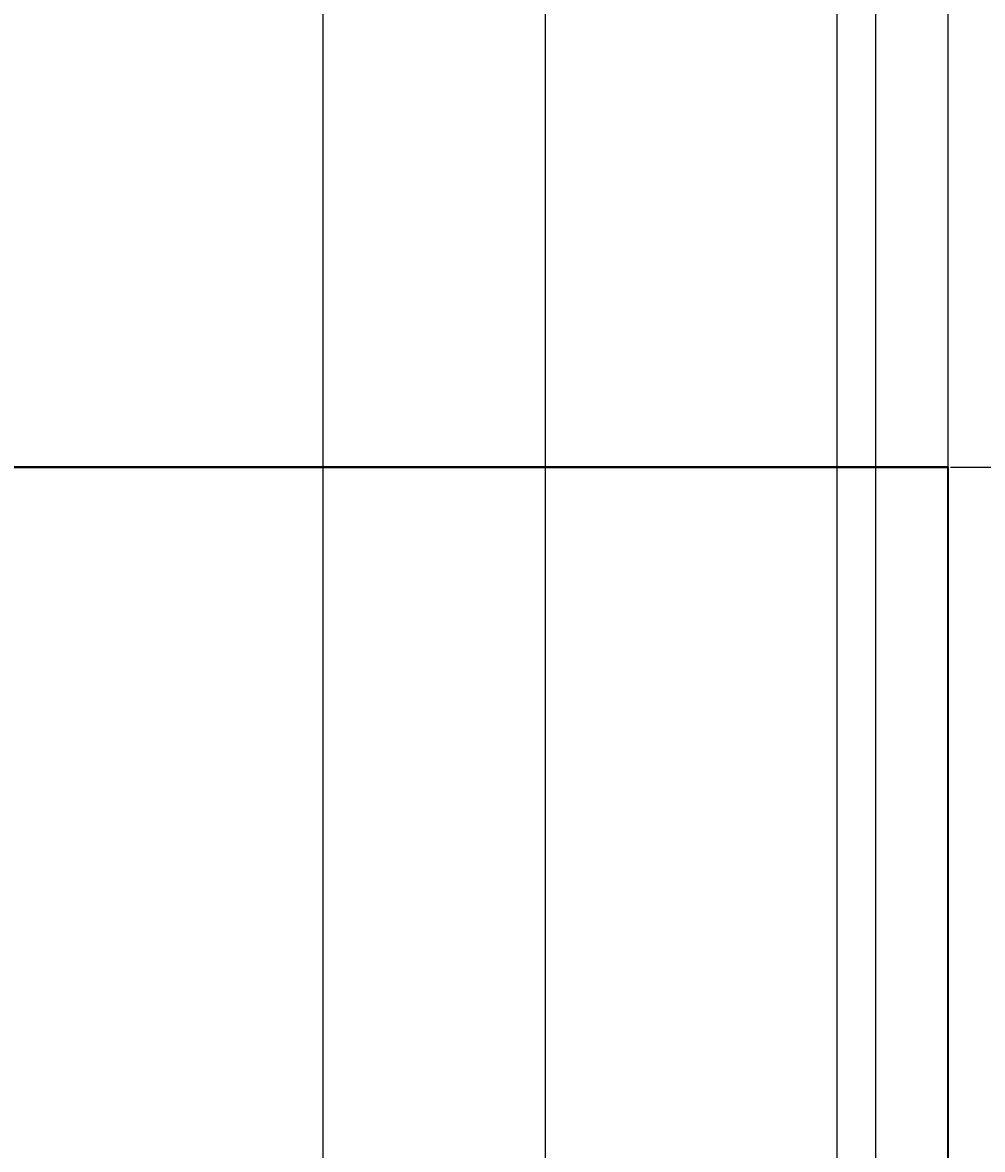
# Model space of a CAD drawing. Units: inches. Extents: x -6 to 289, y -8 to 323.
# Tile 95 of 107: x 222 to 248, y 229 to 259. Entities that reach past the tile are written whole.
import ezdxf

# ---------------------------------------------------------------- set-up
doc = ezdxf.new("R2010")
doc.units = ezdxf.units.IN
doc.header["$MEASUREMENT"] = 0
doc.layers.add('A-ANNO-DIMS', color=2, linetype='Continuous', lineweight=18)
doc.layers.add('A-ELEV', color=7, linetype='Continuous', lineweight=35)
doc.styles.get("Standard").update_dxf_attribs({"font": 'arial.ttf'})
doc.dimstyles.get("Standard").update_dxf_attribs({"dimtxt": 0.18, "dimasz": 0.18, "dimexe": 0.18, "dimexo": 0.0625, "dimgap": 0.09, "dimtad": 0, "dimtih": 1, "dimtoh": 1, "dimdec": 4, "dimzin": 0, "dimdsep": 46, "dimtxsty": 'Standard', "dimcen": 0.09, "dimadec": 0, "dimazin": 0, "dimtfac": 1, "dimtdec": 4, "dimtofl": 0, "dimtmove": 0, "dimatfit": 3, "dimfxl": 1, "dimtolj": 1, "dimtzin": 0, "dimarcsym": 0})

# ---------------------------------------------------------------- blocks, each defined once
blk = doc.blocks.new('*D13')
at = {"layer": 'A-ANNO-DIMS', "color": 0, "lineweight": -2, "transparency": 16777216}
for p, q in [((188.292, 226.951), (188.292, 322.969)), ((236.292, 226.951), (236.292, 322.969)), ((188.472, 322.789), (212.069, 322.789)), ((236.112, 322.789), (212.515, 322.789))]:
    blk.add_line(p, q, dxfattribs=at)
at = {"layer": 'A-ANNO-DIMS', "color": 0, "transparency": 16777216}
for points in [[(188.472, 322.819), (188.472, 322.759), (188.292, 322.789)], [(236.112, 322.819), (236.112, 322.759), (236.292, 322.789)]]:
    blk.add_solid(points, dxfattribs=at)
at = {"layer": 'Defpoints', "color": 0, "transparency": 16777216}
for p in [(236.292, 322.789), (188.292, 226.889), (236.292, 226.889)]:
    blk.add_point(p, dxfattribs=at)
at = {"layer": 'A-ANNO-DIMS', "color": 0, "transparency": 16777216, "insert": (212.292, 322.789), "char_height": 0.18, "attachment_point": 5}
blk.add_mtext('\\A1;48', dxfattribs=at)
blk = doc.blocks.new('*D14')
at = {"layer": 'A-ANNO-DIMS', "color": 0, "lineweight": -2, "transparency": 16777216}
for p, q in [((236.292, 226.951), (236.292, 322.969)), ((247.164, 162.411), (247.164, 322.969)), ((236.472, 322.789), (241.274, 322.789)), ((246.984, 322.789), (242.182, 322.789))]:
    blk.add_line(p, q, dxfattribs=at)
at = {"layer": 'A-ANNO-DIMS', "color": 0, "transparency": 16777216}
for points in [[(236.472, 322.819), (236.472, 322.759), (236.292, 322.789)], [(246.984, 322.819), (246.984, 322.759), (247.164, 322.789)]]:
    blk.add_solid(points, dxfattribs=at)
at = {"layer": 'Defpoints', "color": 0, "transparency": 16777216}
for p in [(247.164, 322.789), (236.292, 226.889), (247.164, 162.348)]:
    blk.add_point(p, dxfattribs=at)
at = {"layer": 'A-ANNO-DIMS', "color": 0, "transparency": 16777216, "insert": (241.728, 322.789), "char_height": 0.18, "attachment_point": 5}
blk.add_mtext('\\A1;10.872', dxfattribs=at)
blk = doc.blocks.new('*D15')
at = {"layer": 'A-ANNO-DIMS', "color": 0, "lineweight": -2, "transparency": 16777216}
for p, q in [((247.164, 162.411), (247.164, 322.969)), ((271.164, 7.351), (271.164, 322.969)), ((247.344, 322.789), (258.944, 322.789)), ((270.984, 322.789), (259.384, 322.789))]:
    blk.add_line(p, q, dxfattribs=at)
at = {"layer": 'A-ANNO-DIMS', "color": 0, "transparency": 16777216}
for points in [[(247.344, 322.819), (247.344, 322.759), (247.164, 322.789)], [(270.984, 322.819), (270.984, 322.759), (271.164, 322.789)]]:
    blk.add_solid(points, dxfattribs=at)
at = {"layer": 'Defpoints', "color": 0, "transparency": 16777216}
for p in [(271.164, 322.789), (247.164, 162.348), (271.164, 7.289)]:
    blk.add_point(p, dxfattribs=at)
at = {"layer": 'A-ANNO-DIMS', "color": 0, "transparency": 16777216, "insert": (259.164, 322.789), "char_height": 0.18, "attachment_point": 5}
blk.add_mtext('\\A1;24', dxfattribs=at)
blk = doc.blocks.new('*D26')
at = {"layer": 'A-ANNO-DIMS', "color": 0, "lineweight": -2, "transparency": 16777216}
for p, q in [((247.226, 247.289), (288.653, 247.289)), ((288.473, 247.109), (288.473, 237.153)), ((288.473, 226.834), (288.473, 236.789)), ((126.946, 226.654), (288.653, 226.654))]:
    blk.add_line(p, q, dxfattribs=at)
at = {"layer": 'A-ANNO-DIMS', "color": 0, "transparency": 16777216}
for points in [[(288.443, 247.109), (288.503, 247.109), (288.473, 247.289)], [(288.443, 226.834), (288.503, 226.834), (288.473, 226.654)]]:
    blk.add_solid(points, dxfattribs=at)
at = {"layer": 'Defpoints', "color": 0, "transparency": 16777216}
for p in [(247.164, 247.289), (288.473, 247.289), (126.883, 226.654)]:
    blk.add_point(p, dxfattribs=at)
at = {"layer": 'A-ANNO-DIMS', "color": 0, "transparency": 16777216, "insert": (288.473, 236.971), "char_height": 0.18, "attachment_point": 5}
blk.add_mtext('\\A1;20.635', dxfattribs=at)
blk = doc.blocks.new('*D27')
at = {"layer": 'A-ANNO-DIMS', "color": 0, "lineweight": -2, "transparency": 16777216}
for p, q in [((19.226, 307.289), (288.653, 307.289)), ((288.473, 307.109), (288.473, 277.471)), ((288.473, 247.469), (288.473, 277.107)), ((247.226, 247.289), (288.653, 247.289))]:
    blk.add_line(p, q, dxfattribs=at)
at = {"layer": 'A-ANNO-DIMS', "color": 0, "transparency": 16777216}
for points in [[(288.443, 307.109), (288.503, 307.109), (288.473, 307.289)], [(288.443, 247.469), (288.503, 247.469), (288.473, 247.289)]]:
    blk.add_solid(points, dxfattribs=at)
at = {"layer": 'Defpoints', "color": 0, "transparency": 16777216}
for p in [(19.164, 307.289), (288.473, 307.289), (247.164, 247.289)]:
    blk.add_point(p, dxfattribs=at)
at = {"layer": 'A-ANNO-DIMS', "color": 0, "transparency": 16777216, "insert": (288.473, 277.289), "char_height": 0.18, "attachment_point": 5}
blk.add_mtext('\\A1;60', dxfattribs=at)
blk = doc.blocks.new('*D80')
at = {"layer": 'A-ANNO-DIMS', "color": 0, "lineweight": -2, "transparency": 16777216}
for p, q in [((188.292, 116.842), (188.292, 322.969)), ((230.292, 116.842), (230.292, 322.969)), ((188.472, 322.789), (209.07, 322.789)), ((230.112, 322.789), (209.513, 322.789))]:
    blk.add_line(p, q, dxfattribs=at)
at = {"layer": 'A-ANNO-DIMS', "color": 0, "transparency": 16777216}
for points in [[(188.472, 322.819), (188.472, 322.759), (188.292, 322.789)], [(230.112, 322.819), (230.112, 322.759), (230.292, 322.789)]]:
    blk.add_solid(points, dxfattribs=at)
at = {"layer": 'Defpoints', "color": 0, "transparency": 16777216}
for p in [(230.292, 322.789), (188.292, 116.779), (230.292, 116.779)]:
    blk.add_point(p, dxfattribs=at)
at = {"layer": 'A-ANNO-DIMS', "color": 0, "transparency": 16777216, "insert": (209.292, 322.789), "char_height": 0.18, "attachment_point": 5}
blk.add_mtext('\\A1;42', dxfattribs=at)
blk = doc.blocks.new('*D81')
at = {"layer": 'A-ANNO-DIMS', "color": 0, "lineweight": -2, "transparency": 16777216}
for p, q in [((230.292, 68.842), (230.292, 322.969)), ((245.215, 66.286), (245.215, 322.969)), ((230.472, 322.789), (237.298, 322.789)), ((245.035, 322.789), (238.208, 322.789))]:
    blk.add_line(p, q, dxfattribs=at)
at = {"layer": 'A-ANNO-DIMS', "color": 0, "transparency": 16777216}
for points in [[(230.472, 322.819), (230.472, 322.759), (230.292, 322.789)], [(245.035, 322.819), (245.035, 322.759), (245.215, 322.789)]]:
    blk.add_solid(points, dxfattribs=at)
at = {"layer": 'Defpoints', "color": 0, "transparency": 16777216}
for p in [(245.215, 322.789), (230.292, 68.779), (245.215, 66.224)]:
    blk.add_point(p, dxfattribs=at)
at = {"layer": 'A-ANNO-DIMS', "color": 0, "transparency": 16777216, "insert": (237.753, 322.789), "char_height": 0.18, "attachment_point": 5}
blk.add_mtext('\\A1;14.923', dxfattribs=at)
blk = doc.blocks.new('*D82')
at = {"layer": 'A-ANNO-DIMS', "color": 0, "lineweight": -2, "transparency": 16777216}
for p, q in [((245.215, 66.286), (245.215, 322.969)), ((272.973, 66.286), (272.973, 322.969)), ((245.395, 322.789), (258.699, 322.789)), ((272.793, 322.789), (259.489, 322.789))]:
    blk.add_line(p, q, dxfattribs=at)
at = {"layer": 'A-ANNO-DIMS', "color": 0, "transparency": 16777216}
for points in [[(245.395, 322.819), (245.395, 322.759), (245.215, 322.789)], [(272.793, 322.819), (272.793, 322.759), (272.973, 322.789)]]:
    blk.add_solid(points, dxfattribs=at)
at = {"layer": 'Defpoints', "color": 0, "transparency": 16777216}
for p in [(272.973, 322.789), (245.215, 66.224), (272.973, 66.224)]:
    blk.add_point(p, dxfattribs=at)
at = {"layer": 'A-ANNO-DIMS', "color": 0, "transparency": 16777216, "insert": (259.094, 322.789), "char_height": 0.18, "attachment_point": 5}
blk.add_mtext('\\A1;27.76', dxfattribs=at)
blk = doc.blocks.new('*D98')
at = {"layer": 'A-ANNO-DIMS', "color": 0, "lineweight": -2, "transparency": 16777216}
for p, q in [((202.741, 159.411), (202.741, 322.969)), ((244.164, 159.411), (244.164, 322.969)), ((202.921, 322.789), (223.056, 322.789)), ((243.984, 322.789), (223.849, 322.789))]:
    blk.add_line(p, q, dxfattribs=at)
at = {"layer": 'A-ANNO-DIMS', "color": 0, "transparency": 16777216}
for points in [[(202.921, 322.819), (202.921, 322.759), (202.741, 322.789)], [(243.984, 322.819), (243.984, 322.759), (244.164, 322.789)]]:
    blk.add_solid(points, dxfattribs=at)
at = {"layer": 'Defpoints', "color": 0, "transparency": 16777216}
for p in [(244.164, 322.789), (202.741, 159.348), (244.164, 159.348)]:
    blk.add_point(p, dxfattribs=at)
at = {"layer": 'A-ANNO-DIMS', "color": 0, "transparency": 16777216, "insert": (223.452, 322.789), "char_height": 0.18, "attachment_point": 5}
blk.add_mtext('\\A1;41.42', dxfattribs=at)
blk = doc.blocks.new('*D99')
at = {"layer": 'A-ANNO-DIMS', "color": 0, "lineweight": -2, "transparency": 16777216}
for p, q in [((244.164, 159.411), (244.164, 322.969)), ((247.164, 162.411), (247.164, 322.969)), ((244.344, 322.789), (245.515, 322.789)), ((246.984, 322.789), (245.813, 322.789))]:
    blk.add_line(p, q, dxfattribs=at)
at = {"layer": 'A-ANNO-DIMS', "color": 0, "transparency": 16777216}
for points in [[(244.344, 322.819), (244.344, 322.759), (244.164, 322.789)], [(246.984, 322.819), (246.984, 322.759), (247.164, 322.789)]]:
    blk.add_solid(points, dxfattribs=at)
at = {"layer": 'Defpoints', "color": 0, "transparency": 16777216}
for p in [(247.164, 322.789), (247.164, 162.348), (244.164, 159.348)]:
    blk.add_point(p, dxfattribs=at)
at = {"layer": 'A-ANNO-DIMS', "color": 0, "transparency": 16777216, "insert": (245.664, 322.789), "char_height": 0.18, "attachment_point": 5}
blk.add_mtext('\\A1;3', dxfattribs=at)
blk = doc.blocks.new('*D100')
at = {"layer": 'A-ANNO-DIMS', "color": 0, "lineweight": -2, "transparency": 16777216}
for p, q in [((247.164, 162.411), (247.164, 322.969)), ((259.164, 139.351), (259.164, 322.969)), ((247.344, 322.789), (252.954, 322.789)), ((258.984, 322.789), (253.373, 322.789))]:
    blk.add_line(p, q, dxfattribs=at)
at = {"layer": 'A-ANNO-DIMS', "color": 0, "transparency": 16777216}
for points in [[(247.344, 322.819), (247.344, 322.759), (247.164, 322.789)], [(258.984, 322.819), (258.984, 322.759), (259.164, 322.789)]]:
    blk.add_solid(points, dxfattribs=at)
at = {"layer": 'Defpoints', "color": 0, "transparency": 16777216}
for p in [(259.164, 322.789), (247.164, 162.348), (259.164, 139.289)]:
    blk.add_point(p, dxfattribs=at)
at = {"layer": 'A-ANNO-DIMS', "color": 0, "transparency": 16777216, "insert": (253.164, 322.789), "char_height": 0.18, "attachment_point": 5}
blk.add_mtext('\\A1;12', dxfattribs=at)
blk = doc.blocks.new('*D113')
at = {"layer": 'A-ANNO-DIMS', "color": 0, "lineweight": -2, "transparency": 16777216}
for p, q in [((271.226, 259.289), (288.653, 259.289)), ((288.473, 259.109), (288.473, 253.469)), ((288.473, 247.469), (288.473, 253.108)), ((247.226, 247.289), (288.653, 247.289))]:
    blk.add_line(p, q, dxfattribs=at)
at = {"layer": 'A-ANNO-DIMS', "color": 0, "transparency": 16777216}
for points in [[(288.443, 259.109), (288.503, 259.109), (288.473, 259.289)], [(288.443, 247.469), (288.503, 247.469), (288.473, 247.289)]]:
    blk.add_solid(points, dxfattribs=at)
at = {"layer": 'Defpoints', "color": 0, "transparency": 16777216}
for p in [(271.164, 259.289), (288.473, 259.289), (247.164, 247.289)]:
    blk.add_point(p, dxfattribs=at)
at = {"layer": 'A-ANNO-DIMS', "color": 0, "transparency": 16777216, "insert": (288.473, 253.289), "char_height": 0.18, "attachment_point": 5}
blk.add_mtext('\\A1;12', dxfattribs=at)

msp = doc.modelspace()

# ---------------------------------------------------------------- linework, layer by layer
at = {"layer": 'A-ELEV'}
for p, q in [((247.1638, 247.2888), (115.1638, 247.2888)), ((115.1638, 247.2888), (247.1638, 247.2888)), ((247.1638, 139.2888), (247.1638, 247.2888))]:
    msp.add_line(p, q, dxfattribs=at)

# ---------------------------------------------------------------- dimensions: what is measured, and where the dimension line sits
at = {"layer": 'A-ANNO-DIMS'}
for base, p1, p2, override, picture, middle in [((236.2918, 322.7888), (188.2918, 226.8887), (236.2918, 226.8887), {"dimdec": 0, "dimlfac": 1, "dimrnd": 0, "dimzin": 0, "dimdsep": 46, "dimlunit": 2}, '*D13', (212.2918, 322.7888)), ((230.2918, 322.7888), (188.2918, 116.7795), (230.2918, 116.7795), {"dimdec": 0, "dimlfac": 1, "dimrnd": 0, "dimzin": 0, "dimdsep": 46, "dimlunit": 2}, '*D80', (209.2918, 322.7888)), ((244.1638, 322.7888), (202.741, 159.3484), (244.1638, 159.3484), {"dimdec": 2, "dimlfac": 1, "dimrnd": 0, "dimzin": 0, "dimdsep": 46, "dimlunit": 2}, '*D98', (223.4524, 322.7888)), ((245.2146, 322.7888), (230.2918, 68.7795), (245.2146, 66.2238), {"dimdec": 3, "dimlfac": 1, "dimrnd": 0, "dimzin": 0, "dimdsep": 46, "dimlunit": 2}, '*D81', (237.7532, 322.7888)), ((247.1638, 322.7888), (236.2918, 226.8887), (247.1638, 162.3484), {"dimdec": 3, "dimlfac": 1, "dimrnd": 0, "dimzin": 0, "dimdsep": 46, "dimlunit": 2}, '*D14', (241.7278, 322.7888)), ((247.1638, 322.7888), (244.1638, 159.3484), (247.1638, 162.3484), {"dimdec": 0, "dimlfac": 1, "dimrnd": 0, "dimzin": 0, "dimdsep": 46, "dimlunit": 2}, '*D99', (245.6638, 322.7888)), ((272.9733, 322.7888), (245.2146, 66.2238), (272.9733, 66.2238), {"dimdec": 2, "dimlfac": 1, "dimrnd": 0, "dimzin": 0, "dimdsep": 46, "dimlunit": 2}, '*D82', (259.0939, 322.7888)), ((271.1638, 322.7888), (247.1638, 162.3484), (271.1638, 7.2888), {"dimdec": 0, "dimlfac": 1, "dimrnd": 0, "dimzin": 0, "dimdsep": 46, "dimlunit": 2}, '*D15', (259.1638, 322.7888)), ((259.1638, 322.7888), (247.1638, 162.3484), (259.1638, 139.2888), {"dimdec": 0, "dimlfac": 1, "dimrnd": 0, "dimzin": 0, "dimdsep": 46, "dimlunit": 2}, '*D100', (253.1638, 322.7888))]:
    dim = msp.add_linear_dim(base=base, p1=p1, p2=p2, dimstyle='Standard', override=override, dxfattribs=at)
    dim.commit()
    dim.dimension.update_dxf_attribs({"geometry": picture, "text_midpoint": middle})
for base, p1, p2, override, picture, middle in [((288.4733, 307.2888), (247.1638, 247.2888), (19.1638, 307.2888), {"dimdec": 0, "dimlfac": 1, "dimrnd": 0, "dimzin": 0, "dimdsep": 46, "dimlunit": 2}, '*D27', (288.4733, 277.2888)), ((288.4733, 259.2888), (247.1638, 247.2888), (271.1638, 259.2888), {"dimdec": 0, "dimlfac": 1, "dimrnd": 0, "dimzin": 0, "dimdsep": 46, "dimlunit": 2}, '*D113', (288.4733, 253.2888)), ((288.4733, 247.2888), (126.8835, 226.654), (247.1638, 247.2888), {"dimdec": 3, "dimlfac": 1, "dimrnd": 0, "dimzin": 0, "dimdsep": 46, "dimlunit": 2}, '*D26', (288.4733, 236.9714))]:
    dim = msp.add_linear_dim(base=base, p1=p1, p2=p2, angle=90, dimstyle='Standard', override=override, dxfattribs=at)
    dim.commit()
    dim.dimension.update_dxf_attribs({"geometry": picture, "text_midpoint": middle})

doc.saveas('drawing.dxf')
